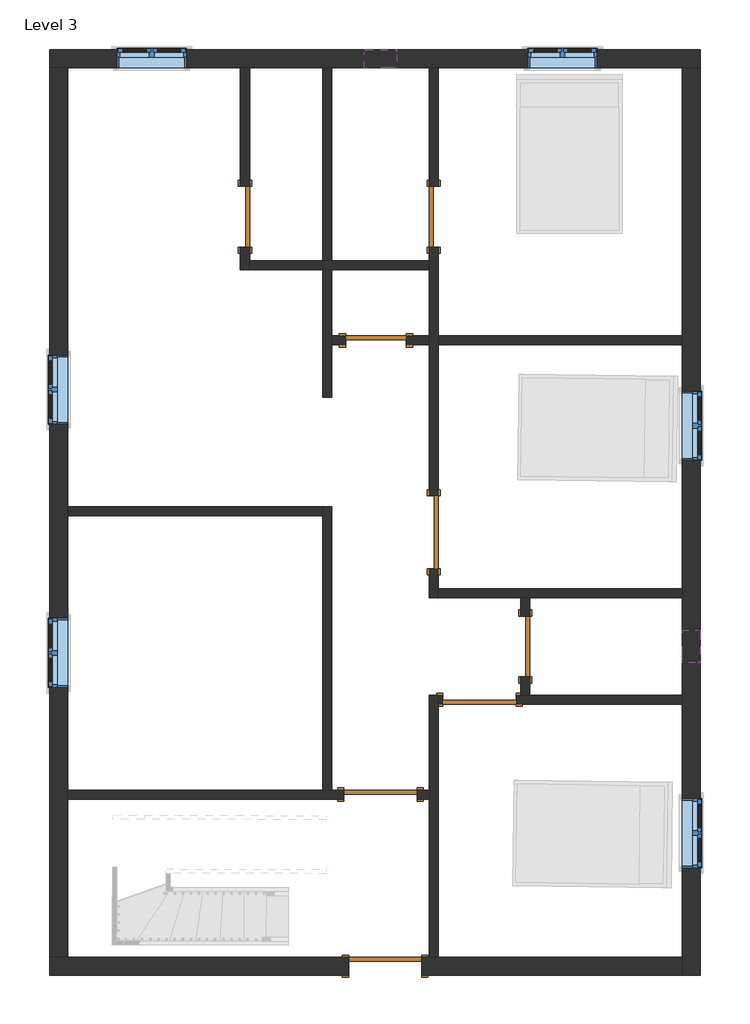
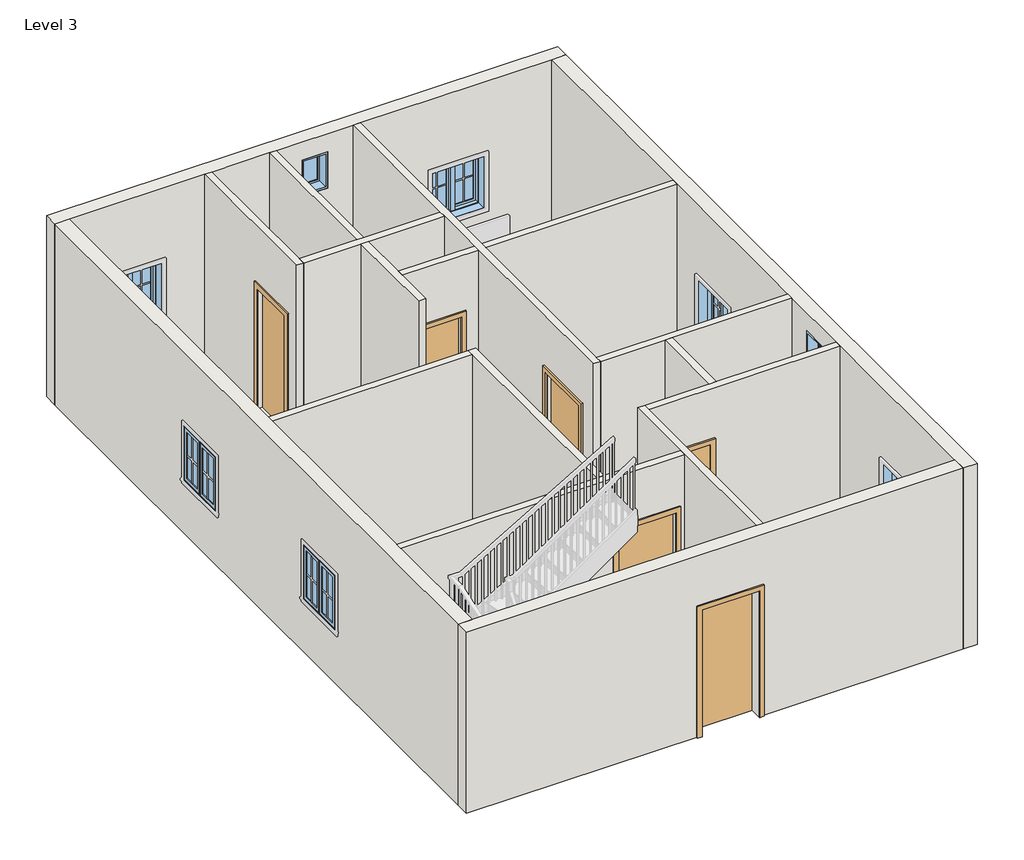
# One storey, part 1 of 3: 17 walls, 8 doors, 8 windows.
"""IFC4 building model written with IfcOpenShell, lengths in millimetres."""

from ifc_helpers import new_model, si_unit, frame, origin, place, context, project, spatial, polyline, outline, extrude, faceted_brep, transform, mapped, element, save
from components import door_d8f5dbb5, door_f2b275c1, door_e5f9f3c4, door_305aa2a5, door_0ca8825f, window_aa618e30, window_339605e1

model = new_model("IFC4")

# Units and contexts
model_context = context("Model", 3, world=origin())
ifc_project = project(units=[si_unit("LENGTHUNIT", "METRE", prefix="MILLI")], contexts=[model_context])

# Site, building, storey
site = spatial("IfcSite", under=ifc_project)
building = spatial("IfcBuilding", under=site)
storey = spatial("IfcBuildingStorey", under=building, Name="Level 3", Elevation=3200.4)

# Doors
placement = place(None, origin())
door_shape = door_d8f5dbb5(model_context)
element("IfcDoor", 1, ObjectType="Single-Flush : 30\" x 80\"", at=placement, inside=storey, context=model_context, shape_type="MappedRepresentation", body=[
    mapped(door_shape, transform((-2883.8867314, 4242.0321212, 3200.4), x_axis=(0.0, -1.0, 0.0), y_axis=(1.0, 0.0, 0.0), z_axis=(0.0, 0.0, 1.0))),
])
door_2_shape = door_f2b275c1(model_context)
element("IfcDoor", 2, ObjectType="Single-Flush : 30\" x 80\"", at=placement, inside=storey, context=model_context, shape_type="MappedRepresentation", body=[
    mapped(door_2_shape, transform((-521.6867314, 4242.0321212, 3200.4), x_axis=(0.0, -1.0, 0.0), y_axis=(1.0, 0.0, 0.0), z_axis=(0.0, 0.0, 1.0))),
])
element("IfcDoor", 3, ObjectType="Single-Flush : 30\" x 80\"", at=placement, inside=storey, context=model_context, shape_type="MappedRepresentation", body=[
    mapped(door_2_shape, transform((-1245.5867314, 2692.6321212, 3200.4), x_axis=(-1.0, 0.0, 0.0), y_axis=(0.0, -1.0, 0.0), z_axis=(0.0, 0.0, 1.0))),
])
element("IfcDoor", 4, ObjectType="Single-Flush : 30\" x 80\"", at=placement, inside=storey, context=model_context, shape_type="MappedRepresentation", body=[
    mapped(door_2_shape, transform((621.3132686, -1136.4178788, 3200.4), x_axis=(0.0, 1.0, 0.0), y_axis=(-1.0, 0.0, 0.0), z_axis=(0.0, 0.0, 1.0))),
])
door_3_shape = door_e5f9f3c4(model_context)
element("IfcDoor", 5, ObjectType="Single-Flush : 36\" x 84\"", at=placement, inside=storey, context=model_context, shape_type="MappedRepresentation", body=[
    mapped(door_3_shape, transform((-521.6867314, 292.3321212, 3200.4), x_axis=(0.0, -1.0, 0.0), y_axis=(1.0, 0.0, 0.0), z_axis=(0.0, 0.0, 1.0))),
])
element("IfcDoor", 6, ObjectType="Single-Flush : 36\" x 84\"", at=placement, inside=storey, context=model_context, shape_type="MappedRepresentation", body=[
    mapped(door_3_shape, transform((-1188.4367314, -2989.1542682, 3200.4), x_axis=(1.0, 0.0, 0.0), y_axis=(0.0, 1.0, 0.0), z_axis=(0.0, 0.0, 1.0))),
])
door_4_shape = door_305aa2a5(model_context)
element("IfcDoor", 7, ObjectType="Single-Flush : 36\" x 84\"", at=placement, inside=storey, context=model_context, shape_type="MappedRepresentation", body=[
    mapped(door_4_shape, transform((49.8132686, -1803.1678788, 3200.4), x_axis=(1.0, 0.0, 0.0), y_axis=(0.0, 1.0, 0.0), z_axis=(0.0, 0.0, 1.0))),
])
door_5_shape = door_0ca8825f(model_context)
element("IfcDoor", 8, ObjectType="Single-Flush : 36\" x 84\"", at=placement, inside=storey, context=model_context, shape_type="MappedRepresentation", body=[
    mapped(door_5_shape, transform((-1131.2867314, -5136.9178788, 3200.4), x_axis=(1.0, 0.0, 0.0), y_axis=(0.0, 1.0, 0.0), z_axis=(0.0, 0.0, 1.0))),
])

# Walls
element("IfcWall", 9, ObjectType="wall4.5\"", at=placement, inside=storey, context=model_context, shape_type="Brep", body=[
    faceted_brep([(-2941.0367314, 3861.0321212, 5232.4), (-2941.0367314, 3861.0321212, 3200.4), (-2941.0367314, 3575.2821212, 3200.4), (-2941.0367314, 3575.2821212, 6248.4), (-2941.0367314, 6102.5821212, 6248.4), (-2941.0367314, 6102.5821212, 3200.4), (-2941.0367314, 4623.0321212, 3200.4), (-2941.0367314, 4623.0321212, 5232.4), (-2826.7367314, 3575.2821212, 3200.4), (-2826.7367314, 3689.5821212, 3200.4), (-2826.7367314, 3861.0321212, 3200.4), (-2826.7367314, 3861.0321212, 5232.4), (-2826.7367314, 4623.0321212, 5232.4), (-2826.7367314, 4623.0321212, 3200.4), (-2826.7367314, 6102.5821212, 3200.4), (-2826.7367314, 6102.5821212, 6248.4), (-2826.7367314, 3689.5821212, 6248.4), (-2826.7367314, 3575.2821212, 6248.4)], [[[0, 1, 2, 3, 4, 5, 6, 7]], [[8, 9, 10, 11, 12, 13, 14, 15, 16, 17]], [[6, 5, 14, 13]], [[2, 1, 10, 9, 8]], [[5, 4, 15, 14]], [[3, 2, 8, 17]], [[11, 10, 1, 0]], [[12, 11, 0, 7]], [[13, 12, 7, 6]], [[4, 3, 17, 16, 15]]]),
])
element("IfcWall", 10, ObjectType="wall4.5\"", at=placement, inside=storey, context=model_context, shape_type="Brep", body=[
    faceted_brep([(-2826.7367314, 3575.2821212, 3200.4), (-1912.3367314, 3575.2821212, 3200.4), (-1798.0367314, 3575.2821212, 3200.4), (-578.8367314, 3575.2821212, 3200.4), (-578.8367314, 3575.2821212, 6248.4), (-1798.0367314, 3575.2821212, 6248.4), (-1912.3367314, 3575.2821212, 6248.4), (-2826.7367314, 3575.2821212, 6248.4), (-2826.7367314, 3689.5821212, 3200.4), (-2826.7367314, 3689.5821212, 6248.4), (-1912.3367314, 3689.5821212, 6248.4), (-1798.0367314, 3689.5821212, 6248.4), (-578.8367314, 3689.5821212, 6248.4), (-578.8367314, 3689.5821212, 3200.4), (-1798.0367314, 3689.5821212, 3200.4), (-1912.3367314, 3689.5821212, 3200.4)], [[[0, 1, 2, 3, 4, 5, 6, 7]], [[8, 9, 10, 11, 12, 13, 14, 15]], [[3, 2, 1, 0, 8, 15, 14, 13]], [[0, 7, 9, 8]], [[4, 3, 13, 12]], [[7, 6, 5, 4, 12, 11, 10, 9]]]),
])
element("IfcWall", 11, ObjectType="wall4.5\"", at=placement, inside=storey, context=model_context, shape_type="SweptSolid", body=[
    extrude(outline(polyline([(-1912.3367314, 3689.5821212), (-1912.3367314, 6102.5821212), (-1798.0367314, 6102.5821212), (-1798.0367314, 3689.5821212), (-1912.3367314, 3689.5821212)])), frame((0.0, 0.0, 3200.4), z_axis=(0.0, 0.0, 1.0), x_axis=(1.0, 0.0, 0.0)), (0.0, 0.0, 1.0), 3048.0),
])
element("IfcWall", 12, ObjectType="wall4.5\"", at=placement, inside=storey, context=model_context, shape_type="Brep", body=[
    faceted_brep([(-578.8367314, -164.8678788, 5334.0), (-578.8367314, -164.8678788, 3200.4), (-578.8367314, -526.8178788, 3200.4), (-578.8367314, -526.8178788, 6248.4), (-578.8367314, 2635.4821212, 6248.4), (-578.8367314, 2749.7821212, 6248.4), (-578.8367314, 3575.2821212, 6248.4), (-578.8367314, 3689.5821212, 6248.4), (-578.8367314, 6102.5821212, 6248.4), (-578.8367314, 6102.5821212, 3200.4), (-578.8367314, 4623.0321212, 3200.4), (-578.8367314, 4623.0321212, 5232.4), (-578.8367314, 3861.0321212, 5232.4), (-578.8367314, 3861.0321212, 3200.4), (-578.8367314, 3689.5821212, 3200.4), (-578.8367314, 3575.2821212, 3200.4), (-578.8367314, 2749.7821212, 3200.4), (-578.8367314, 2635.4821212, 3200.4), (-578.8367314, 749.5321212, 3200.4), (-578.8367314, 749.5321212, 5334.0), (-464.5367314, -526.8178788, 3200.4), (-464.5367314, -412.5178788, 3200.4), (-464.5367314, -164.8678788, 3200.4), (-464.5367314, -164.8678788, 5334.0), (-464.5367314, 749.5321212, 5334.0), (-464.5367314, 749.5321212, 3200.4), (-464.5367314, 2635.4821212, 3200.4), (-464.5367314, 2749.7821212, 3200.4), (-464.5367314, 3861.0321212, 3200.4), (-464.5367314, 3861.0321212, 5232.4), (-464.5367314, 4623.0321212, 5232.4), (-464.5367314, 4623.0321212, 3200.4), (-464.5367314, 6102.5821212, 3200.4), (-464.5367314, 6102.5821212, 6248.4), (-464.5367314, 2749.7821212, 6248.4), (-464.5367314, 2635.4821212, 6248.4), (-464.5367314, -412.5178788, 6248.4), (-464.5367314, -526.8178788, 6248.4)], [[[0, 1, 2, 3, 4, 5, 6, 7, 8, 9, 10, 11, 12, 13, 14, 15, 16, 17, 18, 19]], [[20, 21, 22, 23, 24, 25, 26, 27, 28, 29, 30, 31, 32, 33, 34, 35, 36, 37]], [[10, 9, 32, 31]], [[2, 1, 22, 21, 20]], [[18, 17, 16, 15, 14, 13, 28, 27, 26, 25]], [[9, 8, 33, 32]], [[3, 2, 20, 37]], [[29, 28, 13, 12]], [[30, 29, 12, 11]], [[31, 30, 11, 10]], [[23, 22, 1, 0]], [[24, 23, 0, 19]], [[25, 24, 19, 18]], [[8, 7, 6, 5, 4, 3, 37, 36, 35, 34, 33]]]),
])
element("IfcWall", 13, ObjectType="wall4.5\"", at=placement, inside=storey, context=model_context, shape_type="Brep", body=[
    faceted_brep([(-464.5367314, -526.8178788, 3200.4), (564.1632686, -526.8178788, 3200.4), (678.4632686, -526.8178788, 3200.4), (2583.4632686, -526.8178788, 3200.4), (2583.4632686, -526.8178788, 6248.4), (678.4632686, -526.8178788, 6248.4), (564.1632686, -526.8178788, 6248.4), (-464.5367314, -526.8178788, 6248.4), (-464.5367314, -412.5178788, 3200.4), (-464.5367314, -412.5178788, 6248.4), (2583.4632686, -412.5178788, 6248.4), (2583.4632686, -412.5178788, 3200.4)], [[[0, 1, 2, 3, 4, 5, 6, 7]], [[8, 9, 10, 11]], [[3, 2, 1, 0, 8, 11]], [[0, 7, 9, 8]], [[4, 3, 11, 10]], [[7, 6, 5, 4, 10, 9]]]),
])
element("IfcWall", 14, ObjectType="wall4.5\"", at=placement, inside=storey, context=model_context, shape_type="SweptSolid", body=[
    extrude(outline(polyline([(2583.4632686, 2749.7821212), (2583.4632686, 2635.4821212), (-464.5367314, 2635.4821212), (-464.5367314, 2749.7821212), (2583.4632686, 2749.7821212)])), frame((0.0, 0.0, 3200.4), z_axis=(0.0, 0.0, 1.0), x_axis=(1.0, 0.0, 0.0)), (0.0, 0.0, 1.0), 3048.0),
    extrude(outline(polyline([(6248.4, -1798.0367314), (3200.4, -1798.0367314), (3200.4, -1626.5867314), (5232.4, -1626.5867314), (5232.4, -864.5867314), (3200.4, -864.5867314), (3200.4, -578.8367314), (6248.4, -578.8367314), (6248.4, -1798.0367314)])), frame((0.0, 2635.4821212, 0.0), z_axis=(0.0, 1.0, 0.0), x_axis=(0.0, 0.0, 1.0)), (0.0, 0.0, 1.0), 114.3),
])
element("IfcWall", 15, ObjectType="wall4.5\"", at=placement, inside=storey, context=model_context, shape_type="Brep", body=[
    faceted_brep([(-1912.3367314, 3575.2821212, 3200.4), (-1912.3367314, 1982.8957318, 3200.4), (-1912.3367314, 1982.8957318, 6248.4), (-1912.3367314, 3575.2821212, 6248.4), (-1798.0367314, 3575.2821212, 3200.4), (-1798.0367314, 3575.2821212, 6248.4), (-1798.0367314, 2749.7821212, 6248.4), (-1798.0367314, 2635.4821212, 6248.4), (-1798.0367314, 1982.8957318, 6248.4), (-1798.0367314, 1982.8957318, 3200.4), (-1798.0367314, 2635.4821212, 3200.4), (-1798.0367314, 2749.7821212, 3200.4)], [[[0, 1, 2, 3]], [[4, 5, 6, 7, 8, 9, 10, 11]], [[1, 0, 4, 11, 10, 9]], [[2, 1, 9, 8]], [[0, 3, 5, 4]], [[3, 2, 8, 7, 6, 5]]]),
])
element("IfcWall", 16, ObjectType="wall4.5\"", at=placement, inside=storey, context=model_context, shape_type="Brep", body=[
    faceted_brep([(-1912.3367314, 611.2957318, 3200.4), (-1912.3367314, 496.9957318, 3200.4), (-1912.3367314, -2932.0042682, 3200.4), (-1912.3367314, -2932.0042682, 6248.4), (-1912.3367314, 496.9957318, 6248.4), (-1912.3367314, 611.2957318, 6248.4), (-1798.0367314, 611.2957318, 3200.4), (-1798.0367314, 611.2957318, 6248.4), (-1798.0367314, -2932.0042682, 6248.4), (-1798.0367314, -2932.0042682, 3200.4)], [[[0, 1, 2, 3, 4, 5]], [[6, 7, 8, 9]], [[2, 1, 0, 6, 9]], [[3, 2, 9, 8]], [[0, 5, 7, 6]], [[5, 4, 3, 8, 7]]]),
])
element("IfcWall", 17, ObjectType="wall4.5\"", at=placement, inside=storey, context=model_context, shape_type="Brep", body=[
    faceted_brep([(-731.2367314, -3046.3042682, 5334.0), (-731.2367314, -3046.3042682, 3200.4), (-578.8367314, -3046.3042682, 3200.4), (-578.8367314, -3046.3042682, 6248.4), (-5100.0367314, -3046.3042682, 6248.4), (-5100.0367314, -3046.3042682, 3200.4), (-1645.6367314, -3046.3042682, 3200.4), (-1645.6367314, -3046.3042682, 5334.0), (-578.8367314, -2932.0042682, 3200.4), (-731.2367314, -2932.0042682, 3200.4), (-731.2367314, -2932.0042682, 5334.0), (-1645.6367314, -2932.0042682, 5334.0), (-1645.6367314, -2932.0042682, 3200.4), (-1798.0367314, -2932.0042682, 3200.4), (-1912.3367314, -2932.0042682, 3200.4), (-5100.0367314, -2932.0042682, 3200.4), (-5100.0367314, -2932.0042682, 6248.4), (-1912.3367314, -2932.0042682, 6248.4), (-1798.0367314, -2932.0042682, 6248.4), (-578.8367314, -2932.0042682, 6248.4)], [[[0, 1, 2, 3, 4, 5, 6, 7]], [[8, 9, 10, 11, 12, 13, 14, 15, 16, 17, 18, 19]], [[6, 5, 15, 14, 13, 12]], [[2, 1, 9, 8]], [[5, 4, 16, 15]], [[3, 2, 8, 19]], [[10, 9, 1, 0]], [[11, 10, 0, 7]], [[12, 11, 7, 6]], [[4, 3, 19, 18, 17, 16]]]),
])
element("IfcWall", 18, ObjectType="wall4.5\"", at=placement, inside=storey, context=model_context, shape_type="Brep", body=[
    faceted_brep([(-464.5367314, -5022.6178788, 3200.4), (-464.5367314, -1860.3178788, 3200.4), (-464.5367314, -1746.0178788, 3200.4), (-464.5367314, -1746.0178788, 6248.4), (-464.5367314, -1860.3178788, 6248.4), (-464.5367314, -5022.6178788, 6248.4), (-578.8367314, -5022.6178788, 3200.4), (-578.8367314, -5022.6178788, 6248.4), (-578.8367314, -3046.3042682, 6248.4), (-578.8367314, -2932.0042682, 6248.4), (-578.8367314, -1746.0178788, 6248.4), (-578.8367314, -1746.0178788, 3200.4), (-578.8367314, -2932.0042682, 3200.4), (-578.8367314, -3046.3042682, 3200.4)], [[[0, 1, 2, 3, 4, 5]], [[6, 7, 8, 9, 10, 11, 12, 13]], [[2, 1, 0, 6, 13, 12, 11]], [[0, 5, 7, 6]], [[3, 2, 11, 10]], [[5, 4, 3, 10, 9, 8, 7]]]),
])
element("IfcWall", 19, ObjectType="wall4.5\"", at=placement, inside=storey, context=model_context, shape_type="Brep", body=[
    faceted_brep([(507.0132686, -1860.3178788, 5334.0), (507.0132686, -1860.3178788, 3200.4), (2583.4632686, -1860.3178788, 3200.4), (2583.4632686, -1860.3178788, 6248.4), (-464.5367314, -1860.3178788, 6248.4), (-464.5367314, -1860.3178788, 3200.4), (-407.3867314, -1860.3178788, 3200.4), (-407.3867314, -1860.3178788, 5334.0), (2583.4632686, -1746.0178788, 3200.4), (678.4632686, -1746.0178788, 3200.4), (564.1632686, -1746.0178788, 3200.4), (507.0132686, -1746.0178788, 3200.4), (507.0132686, -1746.0178788, 5334.0), (-407.3867314, -1746.0178788, 5334.0), (-407.3867314, -1746.0178788, 3200.4), (-464.5367314, -1746.0178788, 3200.4), (-464.5367314, -1746.0178788, 6248.4), (564.1632686, -1746.0178788, 6248.4), (678.4632686, -1746.0178788, 6248.4), (2583.4632686, -1746.0178788, 6248.4)], [[[0, 1, 2, 3, 4, 5, 6, 7]], [[8, 9, 10, 11, 12, 13, 14, 15, 16, 17, 18, 19]], [[6, 5, 15, 14]], [[2, 1, 11, 10, 9, 8]], [[5, 4, 16, 15]], [[3, 2, 8, 19]], [[12, 11, 1, 0]], [[13, 12, 0, 7]], [[14, 13, 7, 6]], [[4, 3, 19, 18, 17, 16]]]),
])
element("IfcWall", 20, ObjectType="wall4.5\"", at=placement, inside=storey, context=model_context, shape_type="SweptSolid", body=[
    extrude(outline(polyline([(-526.8178788, 3200.4), (-755.4178788, 3200.4), (-755.4178788, 5232.4), (-1517.4178788, 5232.4), (-1517.4178788, 3200.4), (-1746.0178788, 3200.4), (-1746.0178788, 6248.4), (-526.8178788, 6248.4), (-526.8178788, 3200.4)])), frame((564.1632686, 0.0, 0.0), z_axis=(1.0, 0.0, 0.0), x_axis=(0.0, 1.0, 0.0)), (0.0, 0.0, 1.0), 114.3),
])
element("IfcWall", 21, ObjectType="wall4.5\"", at=placement, inside=storey, context=model_context, shape_type="SweptSolid", body=[
    extrude(outline(polyline([(-5100.0367314, 611.2957318), (-1912.3367314, 611.2957318), (-1912.3367314, 496.9957318), (-5100.0367314, 496.9957318), (-5100.0367314, 611.2957318)])), frame((0.0, 0.0, 3200.4), z_axis=(0.0, 0.0, 1.0), x_axis=(1.0, 0.0, 0.0)), (0.0, 0.0, 1.0), 3048.0),
])
element("IfcWall", 22, ObjectType="wall9\"", at=placement, inside=storey, context=model_context, shape_type="Brep", body=[
    faceted_brep([(-5328.6367314, 6102.5821212, 3200.4), (-5100.0367314, 6102.5821212, 3200.4), (-2941.0367314, 6102.5821212, 3200.4), (-2826.7367314, 6102.5821212, 3200.4), (-1912.3367314, 6102.5821212, 3200.4), (-1798.0367314, 6102.5821212, 3200.4), (-578.8367314, 6102.5821212, 3200.4), (-464.5367314, 6102.5821212, 3200.4), (2583.4632686, 6102.5821212, 3200.4), (2812.0632686, 6102.5821212, 3200.4), (2812.0632686, 6102.5821212, 6248.4), (2583.4632686, 6102.5821212, 6248.4), (-464.5367314, 6102.5821212, 6248.4), (-578.8367314, 6102.5821212, 6248.4), (-1798.0367314, 6102.5821212, 6248.4), (-1912.3367314, 6102.5821212, 6248.4), (-2826.7367314, 6102.5821212, 6248.4), (-2941.0367314, 6102.5821212, 6248.4), (-5100.0367314, 6102.5821212, 6248.4), (-5328.6367314, 6102.5821212, 6248.4), (-985.2367314, 6102.5821212, 5943.6), (-985.2367314, 6102.5821212, 5334.0), (-1391.6367314, 6102.5821212, 5334.0), (-1391.6367314, 6102.5821212, 5943.6), (1519.8382686, 6102.5821212, 5029.2), (1519.8382686, 6102.5821212, 4114.8), (656.2382686, 6102.5821212, 4114.8), (656.2382686, 6102.5821212, 5029.2), (-3617.3117314, 6102.5821212, 5029.2), (-3617.3117314, 6102.5821212, 4114.8), (-4480.9117314, 6102.5821212, 4114.8), (-4480.9117314, 6102.5821212, 5029.2), (-5328.6367314, 6331.1821212, 3200.4), (-5328.6367314, 6331.1821212, 6248.4), (2812.0632686, 6331.1821212, 6248.4), (2812.0632686, 6331.1821212, 3200.4), (-985.2367314, 6331.1821212, 5943.6), (-1391.6367314, 6331.1821212, 5943.6), (-1391.6367314, 6331.1821212, 5334.0), (-985.2367314, 6331.1821212, 5334.0), (1519.8382686, 6331.1821212, 5029.2), (656.2382686, 6331.1821212, 5029.2), (656.2382686, 6331.1821212, 4114.8), (1519.8382686, 6331.1821212, 4114.8), (-3617.3117314, 6331.1821212, 5029.2), (-4480.9117314, 6331.1821212, 5029.2), (-4480.9117314, 6331.1821212, 4114.8), (-3617.3117314, 6331.1821212, 4114.8)], [[[0, 1, 2, 3, 4, 5, 6, 7, 8, 9, 10, 11, 12, 13, 14, 15, 16, 17, 18, 19], [20, 21, 22, 23], [24, 25, 26, 27], [28, 29, 30, 31]], [[32, 33, 34, 35], [36, 37, 38, 39], [40, 41, 42, 43], [44, 45, 46, 47]], [[9, 8, 7, 6, 5, 4, 3, 2, 1, 0, 32, 35]], [[10, 9, 35, 34]], [[0, 19, 33, 32]], [[21, 20, 36, 39]], [[22, 21, 39, 38]], [[23, 22, 38, 37]], [[20, 23, 37, 36]], [[25, 24, 40, 43]], [[26, 25, 43, 42]], [[27, 26, 42, 41]], [[24, 27, 41, 40]], [[29, 28, 44, 47]], [[30, 29, 47, 46]], [[31, 30, 46, 45]], [[28, 31, 45, 44]], [[19, 18, 17, 16, 15, 14, 13, 12, 11, 10, 34, 33]]]),
])
element("IfcWall", 23, ObjectType="wall9\"", at=placement, inside=storey, context=model_context, shape_type="Brep", body=[
    faceted_brep([(2583.4632686, 6102.5821212, 3200.4), (2583.4632686, 2749.7821212, 3200.4), (2583.4632686, 2635.4821212, 3200.4), (2583.4632686, -412.5178788, 3200.4), (2583.4632686, -526.8178788, 3200.4), (2583.4632686, -1746.0178788, 3200.4), (2583.4632686, -1860.3178788, 3200.4), (2583.4632686, -5022.6178788, 3200.4), (2583.4632686, -5251.2178788, 3200.4), (2583.4632686, -5251.2178788, 6248.4), (2583.4632686, -5022.6178788, 6248.4), (2583.4632686, -1860.3178788, 6248.4), (2583.4632686, -1746.0178788, 6248.4), (2583.4632686, -526.8178788, 6248.4), (2583.4632686, -412.5178788, 6248.4), (2583.4632686, 2635.4821212, 6248.4), (2583.4632686, 2749.7821212, 6248.4), (2583.4632686, 6102.5821212, 6248.4), (2583.4632686, -1339.6178788, 5943.6), (2583.4632686, -1339.6178788, 5334.0), (2583.4632686, -933.2178788, 5334.0), (2583.4632686, -933.2178788, 5943.6), (2583.4632686, 1194.0321212, 5029.2), (2583.4632686, 1194.0321212, 4114.8), (2583.4632686, 2057.6321212, 4114.8), (2583.4632686, 2057.6321212, 5029.2), (2583.4632686, -3901.8428788, 5029.2), (2583.4632686, -3901.8428788, 4114.8), (2583.4632686, -3038.2428788, 4114.8), (2583.4632686, -3038.2428788, 5029.2), (2812.0632686, 6102.5821212, 3200.4), (2812.0632686, 6102.5821212, 6248.4), (2812.0632686, -5251.2178788, 6248.4), (2812.0632686, -5251.2178788, 3200.4), (2812.0632686, -1339.6178788, 5943.6), (2812.0632686, -933.2178788, 5943.6), (2812.0632686, -933.2178788, 5334.0), (2812.0632686, -1339.6178788, 5334.0), (2812.0632686, 1194.0321212, 5029.2), (2812.0632686, 2057.6321212, 5029.2), (2812.0632686, 2057.6321212, 4114.8), (2812.0632686, 1194.0321212, 4114.8), (2812.0632686, -3901.8428788, 5029.2), (2812.0632686, -3038.2428788, 5029.2), (2812.0632686, -3038.2428788, 4114.8), (2812.0632686, -3901.8428788, 4114.8)], [[[0, 1, 2, 3, 4, 5, 6, 7, 8, 9, 10, 11, 12, 13, 14, 15, 16, 17], [18, 19, 20, 21], [22, 23, 24, 25], [26, 27, 28, 29]], [[30, 31, 32, 33], [34, 35, 36, 37], [38, 39, 40, 41], [42, 43, 44, 45]], [[8, 7, 6, 5, 4, 3, 2, 1, 0, 30, 33]], [[0, 17, 31, 30]], [[9, 8, 33, 32]], [[19, 18, 34, 37]], [[20, 19, 37, 36]], [[21, 20, 36, 35]], [[18, 21, 35, 34]], [[23, 22, 38, 41]], [[24, 23, 41, 40]], [[25, 24, 40, 39]], [[22, 25, 39, 38]], [[27, 26, 42, 45]], [[28, 27, 45, 44]], [[29, 28, 44, 43]], [[26, 29, 43, 42]], [[17, 16, 15, 14, 13, 12, 11, 10, 9, 32, 31]]]),
])
element("IfcWall", 24, ObjectType="wall9\"", at=placement, inside=storey, context=model_context, shape_type="Brep", body=[
    faceted_brep([(2583.4632686, -5022.6178788, 3200.4), (-464.5367314, -5022.6178788, 3200.4), (-578.8367314, -5022.6178788, 3200.4), (-674.0867314, -5022.6178788, 3200.4), (-674.0867314, -5022.6178788, 5334.0), (-1588.4867314, -5022.6178788, 5334.0), (-1588.4867314, -5022.6178788, 3200.4), (-5100.0367314, -5022.6178788, 3200.4), (-5328.6367314, -5022.6178788, 3200.4), (-5328.6367314, -5022.6178788, 6248.4), (-5100.0367314, -5022.6178788, 6248.4), (-578.8367314, -5022.6178788, 6248.4), (-464.5367314, -5022.6178788, 6248.4), (2583.4632686, -5022.6178788, 6248.4), (-674.0867314, -5251.2178788, 5334.0), (-674.0867314, -5251.2178788, 3200.4), (2583.4632686, -5251.2178788, 3200.4), (2583.4632686, -5251.2178788, 6248.4), (-5328.6367314, -5251.2178788, 6248.4), (-5328.6367314, -5251.2178788, 3200.4), (-1588.4867314, -5251.2178788, 3200.4), (-1588.4867314, -5251.2178788, 5334.0)], [[[0, 1, 2, 3, 4, 5, 6, 7, 8, 9, 10, 11, 12, 13]], [[14, 15, 16, 17, 18, 19, 20, 21]], [[20, 19, 8, 7, 6]], [[16, 15, 3, 2, 1, 0]], [[0, 13, 17, 16]], [[9, 8, 19, 18]], [[4, 3, 15, 14]], [[5, 4, 14, 21]], [[6, 5, 21, 20]], [[13, 12, 11, 10, 9, 18, 17]]]),
])
element("IfcWall", 25, ObjectType="wall9\"", at=placement, inside=storey, context=model_context, shape_type="Brep", body=[
    faceted_brep([(-5328.6367314, 6102.5821212, 3200.4), (-5328.6367314, -5022.6178788, 3200.4), (-5328.6367314, -5022.6178788, 6248.4), (-5328.6367314, 6102.5821212, 6248.4), (-5328.6367314, 2509.9457318, 5029.2), (-5328.6367314, 1646.3457318, 5029.2), (-5328.6367314, 1646.3457318, 4114.8), (-5328.6367314, 2509.9457318, 4114.8), (-5328.6367314, -785.7042682, 5029.2), (-5328.6367314, -1649.3042682, 5029.2), (-5328.6367314, -1649.3042682, 4114.8), (-5328.6367314, -785.7042682, 4114.8), (-5100.0367314, 6102.5821212, 3200.4), (-5100.0367314, 6102.5821212, 6248.4), (-5100.0367314, 611.2957318, 6248.4), (-5100.0367314, 496.9957318, 6248.4), (-5100.0367314, -2932.0042682, 6248.4), (-5100.0367314, -3046.3042682, 6248.4), (-5100.0367314, -5022.6178788, 6248.4), (-5100.0367314, -5022.6178788, 3200.4), (-5100.0367314, -3046.3042682, 3200.4), (-5100.0367314, -2932.0042682, 3200.4), (-5100.0367314, 496.9957318, 3200.4), (-5100.0367314, 611.2957318, 3200.4), (-5100.0367314, 2509.9457318, 5029.2), (-5100.0367314, 2509.9457318, 4114.8), (-5100.0367314, 1646.3457318, 4114.8), (-5100.0367314, 1646.3457318, 5029.2), (-5100.0367314, -785.7042682, 5029.2), (-5100.0367314, -785.7042682, 4114.8), (-5100.0367314, -1649.3042682, 4114.8), (-5100.0367314, -1649.3042682, 5029.2)], [[[0, 1, 2, 3], [4, 5, 6, 7], [8, 9, 10, 11]], [[12, 13, 14, 15, 16, 17, 18, 19, 20, 21, 22, 23], [24, 25, 26, 27], [28, 29, 30, 31]], [[1, 0, 12, 23, 22, 21, 20, 19]], [[0, 3, 13, 12]], [[2, 1, 19, 18]], [[25, 24, 4, 7]], [[26, 25, 7, 6]], [[27, 26, 6, 5]], [[24, 27, 5, 4]], [[29, 28, 8, 11]], [[30, 29, 11, 10]], [[31, 30, 10, 9]], [[28, 31, 9, 8]], [[3, 2, 18, 17, 16, 15, 14, 13]]]),
])

# Windows
window_shape = window_aa618e30(model_context)
element("IfcWindow", 26, ObjectType="Fixed : 16\" x 24\"", at=placement, inside=storey, context=model_context, shape_type="MappedRepresentation", body=[
    mapped(window_shape, transform((-1150.3367314, 6216.8821212, 4419.6), x_axis=(1.0, 0.0, 0.0), y_axis=(0.0, 1.0, 0.0), z_axis=(0.0, 0.0, 1.0))),
])
element("IfcWindow", 27, ObjectType="Fixed : 16\" x 24\"", at=placement, inside=storey, context=model_context, shape_type="MappedRepresentation", body=[
    mapped(window_shape, transform((2697.7632686, -1174.5178788, 4419.6), x_axis=(0.0, -1.0, 0.0), y_axis=(1.0, 0.0, 0.0), z_axis=(0.0, 0.0, 1.0))),
])
window_2_shape = window_339605e1(model_context)
element("IfcWindow", 28, ObjectType="Window-Casement-Double : 34\" x 36\"", at=placement, inside=storey, context=model_context, shape_type="MappedRepresentation", body=[
    mapped(window_2_shape, transform((1088.0382686, 6216.8821212, 3200.4), x_axis=(1.0, 0.0, 0.0), y_axis=(0.0, 1.0, 0.0), z_axis=(0.0, 0.0, 1.0))),
])
element("IfcWindow", 29, ObjectType="Window-Casement-Double : 34\" x 36\"", at=placement, inside=storey, context=model_context, shape_type="MappedRepresentation", body=[
    mapped(window_2_shape, transform((2697.7632686, 1625.8321212, 3200.4), x_axis=(0.0, -1.0, 0.0), y_axis=(1.0, 0.0, 0.0), z_axis=(0.0, 0.0, 1.0))),
])
element("IfcWindow", 30, ObjectType="Window-Casement-Double : 34\" x 36\"", at=placement, inside=storey, context=model_context, shape_type="MappedRepresentation", body=[
    mapped(window_2_shape, transform((2697.7632686, -3470.0428788, 3200.4), x_axis=(0.0, -1.0, 0.0), y_axis=(1.0, 0.0, 0.0), z_axis=(0.0, 0.0, 1.0))),
])
element("IfcWindow", 31, ObjectType="Window-Casement-Double : 34\" x 36\"", at=placement, inside=storey, context=model_context, shape_type="MappedRepresentation", body=[
    mapped(window_2_shape, transform((-4049.1117314, 6216.8821212, 3200.4), x_axis=(1.0, 0.0, 0.0), y_axis=(0.0, 1.0, 0.0), z_axis=(0.0, 0.0, 1.0))),
])
element("IfcWindow", 32, ObjectType="Window-Casement-Double : 34\" x 36\"", at=placement, inside=storey, context=model_context, shape_type="MappedRepresentation", body=[
    mapped(window_2_shape, transform((-5214.3367314, 2078.1457318, 3200.4), x_axis=(0.0, 1.0, 0.0), y_axis=(-1.0, 0.0, 0.0), z_axis=(0.0, 0.0, 1.0))),
])
element("IfcWindow", 33, ObjectType="Window-Casement-Double : 34\" x 36\"", at=placement, inside=storey, context=model_context, shape_type="MappedRepresentation", body=[
    mapped(window_2_shape, transform((-5214.3367314, -1217.5042682, 3200.4), x_axis=(0.0, 1.0, 0.0), y_axis=(-1.0, 0.0, 0.0), z_axis=(0.0, 0.0, 1.0))),
])

save(model, "model.ifc")

# Revit data of these elements
# Type "Single-Flush : 30\" x 80\""
#   Type Mark = "5"
#   Construction Type Id = "MDOOR"
#   Assembly Code = "C1020"
#   Analytic Construction = "Metal"
#   Thickness = 0' - 2"
#   Heat Transfer Coefficient (U) = 0.651978 BTU/(h·ft²·°F)
#   Height = 6' - 8"
#   Trim Projection Ext = 0' - 1"
#   Trim Projection Int = 0' - 1"
#   Trim Width = 0' - 3"
#   Width = 2' - 6"
#   Define Thermal Properties by = 1
#   Define Thermal Properties by = 1
#   Door Material = Door - Panel
#   Frame Material = Door - Frame
#   Visual Light Transmittance = 0
#   Solar Heat Gain Coefficient = 0
#   Function = (empty or 0)
#   Wall Closure = (empty or 0)
# Type "Single-Flush : 36\" x 84\""
#   Type Mark = "1"
#   Construction Type Id = "MDOOR"
#   Assembly Code = "C1020"
#   Analytic Construction = "Metal"
#   Thickness = 0' - 2"
#   Heat Transfer Coefficient (U) = 0.651978 BTU/(h·ft²·°F)
#   Height = 7' - 0"
#   Trim Projection Ext = 0' - 1"
#   Trim Projection Int = 0' - 1"
#   Trim Width = 0' - 3"
#   Width = 3' - 0"
#   Define Thermal Properties by = 1
#   Define Thermal Properties by = 1
#   Door Material = Door - Panel
#   Frame Material = Door - Frame
#   Visual Light Transmittance = 0
#   Solar Heat Gain Coefficient = 0
#   Function = (empty or 0)
#   Wall Closure = (empty or 0)
# Type "wall4.5\""
#   Assembly Code = "B2010"
#   Layers, outside or top first: 0' - 4 1/2" no material (function 1)
# Type "wall9\""
#   Assembly Code = "B2010"
#   Layers, outside or top first: 0' - 9" no material (function 1)
# Type "Fixed : 16\" x 24\""
#   Type Mark = "4"
#   Construction Type Id = "GSP4R"
#   Assembly Code = "B2020100"
#   Analytic Construction = "1/8 in Pilkington single glazing"
#   Visual Light Transmittance = 0.9
#   Solar Heat Gain Coefficient = 0.78
#   Heat Transfer Coefficient (U) = 0.6496 BTU/(h·ft²·°F)
#   Height = 2' - 0"
#   Default Sill Height = 3' - 0"
#   Width = 1' - 4"
#   Window Inset = 0' - 0 3/4"
#   Define Thermal Properties by = 1
#   Define Thermal Properties by = 1
#   Glass Pane Material = Glass
#   Sash Material = Sash
#   Wall Closure = (empty or 0)
# Type "Window-Casement-Double : 34\" x 36\""
#   Type Mark = "14"
#   Fire Rating = "0.5h"
#   Assembly Code = "B2020100"
#   Analytic Construction = "Double glazing - domestic"
#   Frame Extension [instance default] = 0' - 0 1/4"
#   Window Inset [instance default] = 0' - 0"
#   Wall Thickness [instance default] = 0' - 6"
#   Interior Wall Closure [instance default] = 0' - 2 1/4"
#   Half Width = 1' - 5"
#   Visual Light Transmittance = 0.81
#   Thermal Resistance (R) = 1.8146 (h·ft²·°F)/BTU
#   Solar Heat Gain Coefficient = 0.76
#   Rough Width = 2' - 10 1/2"
#   Rough Height = 3' - 0 1/2"
#   Height = 3' - 0"
#   Heat Transfer Coefficient (U) = 0.5511 BTU/(h·ft²·°F)
#   Exterior Wall Closure [instance default] = 0' - 1 1/4"
#   Extension Jamb [instance default] = 0' - 2 1/4"
#   Default Sill Height = 3' - 0"
#   Width = 2' - 10"
#   Define Thermal Properties by = 0
#   Muntin Visibility = yes
#   Interior Trim Visibility [instance default] = yes
#   Exterior Trim Visibility [instance default] = yes
#   Extension Jamb Visibility [instance default] = yes
#   Interior Trim Material = Wood - Stained
#   Muntin Pattern = Muntin Pattern_2x2 : Muntin Pattern_2x2
#   Interior Trim = Trim-Window-Interior-Flat : Picture Frame
#   Interior Frame Material = Wood - Stained
#   Glass Panel Material = Glass
#   Exterior Trim Material = Clad - White
#   Exterior Trim = Trim-Window-Exterior-Flat : with Sill
#   Exterior Frame Material = Clad - White
#   Wall Closure = (empty or 0)
# Elements 1, 2, 3, 4 (IfcDoor, "Single-Flush : 30\" x 80\"")
#   Phase Created = New Construction
#   Materials on its faces: "Door - Frame", "Door - Panel"
# Elements 5, 6, 7, 8 (IfcDoor, "Single-Flush : 36\" x 84\"")
#   Phase Created = New Construction
#   Materials on its faces: "Door - Frame", "Door - Panel"
# Elements 9, 10, 11, 12, 13, 14, 15, 16, 17, 18, 19, 20, 21 (IfcWall, "wall4.5\"")
#   Top Offset = 0' - 0"
#   Base Offset = 0' - 0"
#   Unconnected Height = 10' - 0"
#   wall height = 10' - 0"
#   Phase Created = New Construction
#   Base Constraint = Level 3
#   Materials on its faces: "Default Wall"
# Elements 22, 23, 24, 25 (IfcWall, "wall9\"")
#   Top Offset = 0' - 0"
#   Base Offset = 0' - 0"
#   Unconnected Height = 10' - 0"
#   wall height = 10' - 0"
#   Phase Created = New Construction
#   Base Constraint = Level 3
#   Materials on its faces: "Default Wall", "Wood Planks"
# Element 26 (IfcWindow, "Fixed : 16\" x 24\"")
#   Mark = "9"
#   Phase Created = New Construction
#   Materials on its faces: "Sash", "Glass"
# Element 27 (IfcWindow, "Fixed : 16\" x 24\"")
#   Mark = "10"
#   Phase Created = New Construction
#   Materials on its faces: "Sash", "Glass"
# Element 28 (IfcWindow, "Window-Casement-Double : 34\" x 36\"")
#   Mark = "11"
#   Window Inset = 0' - 0"
#   Interior Wall Closure = 0' - 2 1/4"
#   Frame Extension = 0' - 0 1/4"
#   Exterior Wall Closure = 0' - 1 1/4"
#   Interior Trim Visibility = yes
#   Exterior Trim Visibility = yes
#   Phase Created = New Construction
#   Materials on its faces: "Wood - Stained", "Glass", "Clad - White"
# Element 29 (IfcWindow, "Window-Casement-Double : 34\" x 36\"")
#   Mark = "12"
#   Window Inset = 0' - 0"
#   Interior Wall Closure = 0' - 2 1/4"
#   Frame Extension = 0' - 0 1/4"
#   Exterior Wall Closure = 0' - 1 1/4"
#   Interior Trim Visibility = yes
#   Exterior Trim Visibility = yes
#   Phase Created = New Construction
#   Materials on its faces: "Wood - Stained", "Glass", "Clad - White"
# Element 30 (IfcWindow, "Window-Casement-Double : 34\" x 36\"")
#   Mark = "13"
#   Window Inset = 0' - 0"
#   Interior Wall Closure = 0' - 2 1/4"
#   Frame Extension = 0' - 0 1/4"
#   Exterior Wall Closure = 0' - 1 1/4"
#   Interior Trim Visibility = yes
#   Exterior Trim Visibility = yes
#   Phase Created = New Construction
#   Materials on its faces: "Wood - Stained", "Glass", "Clad - White"
# Element 31 (IfcWindow, "Window-Casement-Double : 34\" x 36\"")
#   Mark = "14"
#   Window Inset = 0' - 0"
#   Interior Wall Closure = 0' - 2 1/4"
#   Frame Extension = 0' - 0 1/4"
#   Exterior Wall Closure = 0' - 1 1/4"
#   Interior Trim Visibility = yes
#   Exterior Trim Visibility = yes
#   Phase Created = New Construction
#   Materials on its faces: "Wood - Stained", "Glass", "Clad - White"
# Element 32 (IfcWindow, "Window-Casement-Double : 34\" x 36\"")
#   Mark = "15"
#   Window Inset = 0' - 0"
#   Interior Wall Closure = 0' - 2 1/4"
#   Frame Extension = 0' - 0 1/4"
#   Exterior Wall Closure = 0' - 1 1/4"
#   Interior Trim Visibility = yes
#   Exterior Trim Visibility = yes
#   Phase Created = New Construction
#   Materials on its faces: "Wood - Stained", "Glass", "Clad - White"
# Element 33 (IfcWindow, "Window-Casement-Double : 34\" x 36\"")
#   Mark = "16"
#   Window Inset = 0' - 0"
#   Interior Wall Closure = 0' - 2 1/4"
#   Frame Extension = 0' - 0 1/4"
#   Exterior Wall Closure = 0' - 1 1/4"
#   Interior Trim Visibility = yes
#   Exterior Trim Visibility = yes
#   Phase Created = New Construction
#   Materials on its faces: "Wood - Stained", "Glass", "Clad - White"
# Materials
#   "Door - Panel": class "Wood", colour RGB 210 159 95, transparency 0, Cost = 0
#   "Door - Frame": colour RGB 118 70 51, transparency 0, Cost = 0
#   "Glass": class "Glass", colour RGB 0 128 192, transparency 0.75, Description = "Soda Lime Glass", Cost = 0
#   "Sash": class "Wood", colour RGB 224 178 126, transparency 0, Cost = 0
#   "Wood - Stained": class "Wood", colour RGB 224 178 126, transparency 0, Cost = 0
#   "Clad - White": class "Wood", colour RGB 242 242 238, transparency 0, Cost = 0
#   "Default Wall": colour RGB 128 128 128, transparency 0, Cost = 0
#   "Wood Planks": class "Wood", colour RGB 193 160 115, transparency 0, Description = "Physical material.", Cost = 0
